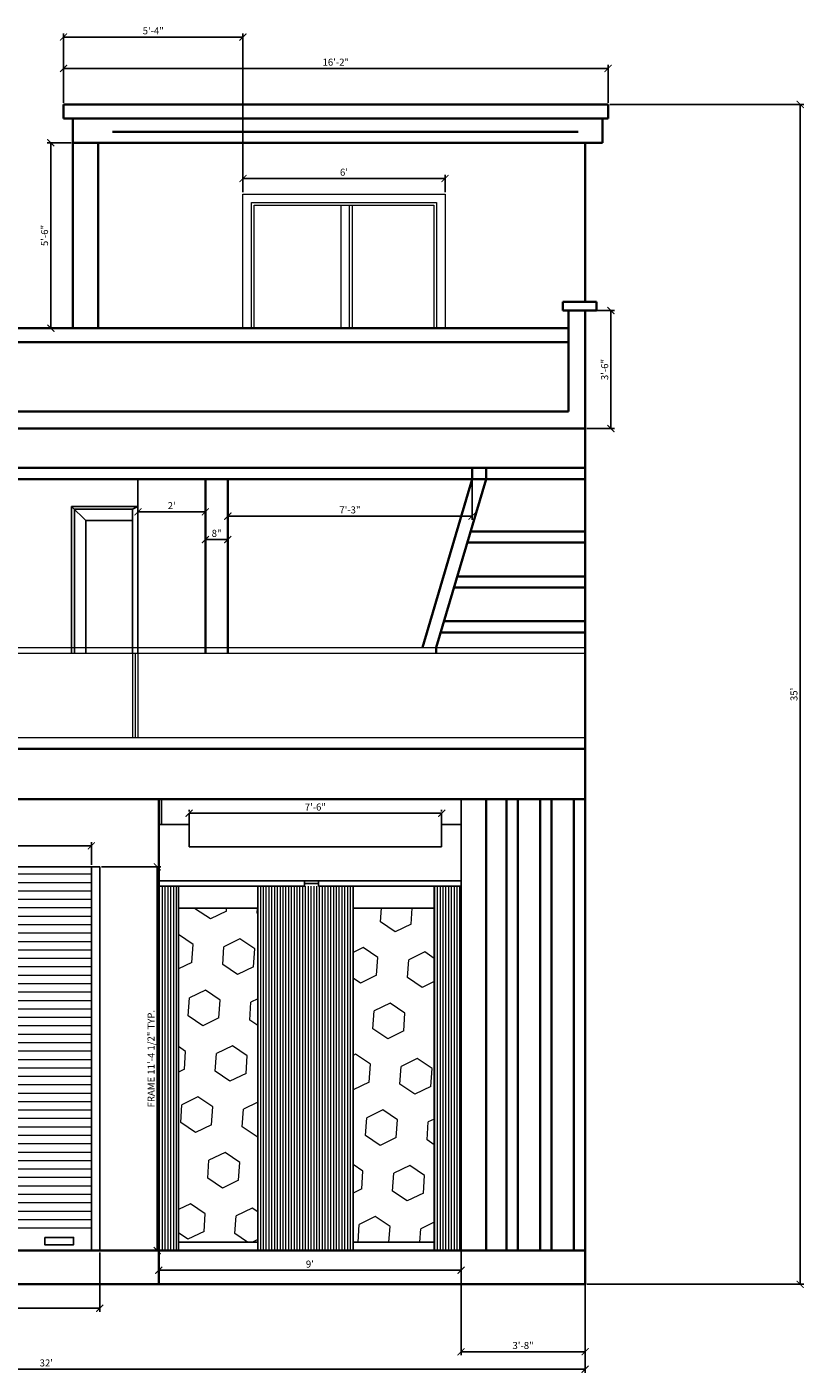
# Model space of a CAD drawing. Units: inches. Extents: x 3122 to 5933, y 1474 to 2995.
# Tile 2 of 12: x 3337 to 3614, y 1583 to 2063. Entities that reach past the tile are written whole.
import ezdxf

# ---------------------------------------------------------------- set-up
doc = ezdxf.new("R2010")
doc.units = ezdxf.units.IN
for name, color, linetype, lineweight in [('A-ANNO-DIMS', 2, 'Continuous', 18), ('A-ELEV', 7, 'Continuous', 35), ('A-ELEV-DOOR', 4, 'Continuous', 25), ('A-ELEV-GLAZ', 4, 'Continuous', 18), ('A-ELEV-PATT', 8, 'Continuous', 13), ('A-ELEV-RAIL', 7, 'Continuous', 18)]:
    doc.layers.add(name, color=color, linetype=linetype, lineweight=lineweight)
doc.styles.get("Standard").update_dxf_attribs({"font": 'arial.ttf'})
doc.dimstyles.new('ISO-25', dxfattribs={"dimtxt": 2.5, "dimasz": 2.5, "dimexe": 1.25, "dimexo": 0.625, "dimtad": 1, "dimdec": 0, "dimlunit": 3, "dimtxsty": 'Standard', "dimblk": 'ARCHTICK', "dimcen": 2.5, "dimadec": 0, "dimazin": 0, "dimtfac": 1, "dimtdec": 0, "dimtmove": 0, "dimatfit": 3, "dimfxl": 1, "dimarcsym": 0})

# ---------------------------------------------------------------- blocks, each defined once
blk = doc.blocks.new('_ArchTick')
at = {"color": 0, "linetype": 'ByBlock', "const_width": 0.15}
blk.add_lwpolyline([(-0.5, -0.5), (0.5, 0.5)], dxfattribs=at)
blk = doc.blocks.new('*D3')
at = {"layer": 'A-ANNO-DIMS', "color": 0, "lineweight": -2, "transparency": 16777216}
for p, q in [((3408.29, 1900.94), (3408.29, 1887.11)), ((3495.29, 1900.94), (3495.29, 1887.11)), ((3408.29, 1888.36), (3495.29, 1888.36))]:
    blk.add_line(p, q, dxfattribs=at)
at = {"layer": 'Defpoints', "color": 0, "transparency": 16777216}
for p in [(3408.29, 1901.56), (3495.29, 1901.56), (3495.29, 1888.36)]:
    blk.add_point(p, dxfattribs=at)
at = {"layer": 'A-ANNO-DIMS', "color": 0, "lineweight": -2, "transparency": 16777216, "xscale": 2.5, "yscale": 2.5, "zscale": 2.5, "rotation": 180}
blk.add_blockref('_ArchTick', (3408.29, 1888.36), dxfattribs=at)
at = {"layer": 'A-ANNO-DIMS', "color": 0, "lineweight": -2, "transparency": 16777216, "xscale": 2.5, "yscale": 2.5, "zscale": 2.5}
blk.add_blockref('_ArchTick', (3495.29, 1888.36), dxfattribs=at)
at = {"layer": 'A-ANNO-DIMS', "color": 0, "transparency": 16777216, "insert": (3451.79, 1890.26), "char_height": 2.5, "attachment_point": 5}
blk.add_mtext('7\'-3"', dxfattribs=at)
blk = doc.blocks.new('*D4')
at = {"layer": 'A-ANNO-DIMS', "color": 0, "lineweight": -2, "transparency": 16777216}
for p, q in [((3400.29, 1900.94), (3400.29, 1878.77)), ((3408.29, 1900.94), (3408.29, 1878.77)), ((3400.29, 1880.02), (3408.29, 1880.02))]:
    blk.add_line(p, q, dxfattribs=at)
at = {"layer": 'Defpoints', "color": 0, "transparency": 16777216}
for p in [(3400.29, 1901.56), (3408.29, 1901.56), (3408.29, 1880.02)]:
    blk.add_point(p, dxfattribs=at)
at = {"layer": 'A-ANNO-DIMS', "color": 0, "lineweight": -2, "transparency": 16777216, "xscale": 2.5, "yscale": 2.5, "zscale": 2.5, "rotation": 180}
blk.add_blockref('_ArchTick', (3400.29, 1880.02), dxfattribs=at)
at = {"layer": 'A-ANNO-DIMS', "color": 0, "lineweight": -2, "transparency": 16777216, "xscale": 2.5, "yscale": 2.5, "zscale": 2.5}
blk.add_blockref('_ArchTick', (3408.29, 1880.02), dxfattribs=at)
at = {"layer": 'A-ANNO-DIMS', "color": 0, "transparency": 16777216, "insert": (3404.29, 1881.92), "char_height": 2.5, "attachment_point": 5}
blk.add_mtext('8"', dxfattribs=at)
blk = doc.blocks.new('*D5')
at = {"layer": 'A-ANNO-DIMS', "color": 0, "lineweight": -2, "transparency": 16777216}
for p, q in [((3376.29, 1900.94), (3376.29, 1888.65)), ((3400.29, 1900.94), (3400.29, 1888.65)), ((3376.29, 1889.9), (3400.29, 1889.9))]:
    blk.add_line(p, q, dxfattribs=at)
at = {"layer": 'Defpoints', "color": 0, "transparency": 16777216}
for p in [(3376.29, 1901.56), (3400.29, 1901.56), (3400.29, 1889.9)]:
    blk.add_point(p, dxfattribs=at)
at = {"layer": 'A-ANNO-DIMS', "color": 0, "lineweight": -2, "transparency": 16777216, "xscale": 2.5, "yscale": 2.5, "zscale": 2.5, "rotation": 180}
blk.add_blockref('_ArchTick', (3376.29, 1889.9), dxfattribs=at)
at = {"layer": 'A-ANNO-DIMS', "color": 0, "lineweight": -2, "transparency": 16777216, "xscale": 2.5, "yscale": 2.5, "zscale": 2.5}
blk.add_blockref('_ArchTick', (3400.29, 1889.9), dxfattribs=at)
at = {"layer": 'A-ANNO-DIMS', "color": 0, "transparency": 16777216, "insert": (3388.29, 1891.78), "char_height": 2.5, "attachment_point": 5}
blk.add_mtext("2'", dxfattribs=at)
blk = doc.blocks.new('*D6')
at = {"layer": 'A-ANNO-DIMS', "color": 0, "lineweight": -2, "transparency": 16777216}
for p, q in [((3413.67, 2003.64), (3413.67, 2009.81)), ((3413.67, 2008.56), (3485.67, 2008.56)), ((3485.67, 2003.64), (3485.67, 2009.81))]:
    blk.add_line(p, q, dxfattribs=at)
at = {"layer": 'Defpoints', "color": 0, "transparency": 16777216}
for p in [(3485.67, 2008.56), (3413.67, 2003.02), (3485.67, 2003.02)]:
    blk.add_point(p, dxfattribs=at)
at = {"layer": 'A-ANNO-DIMS', "color": 0, "lineweight": -2, "transparency": 16777216, "xscale": 2.5, "yscale": 2.5, "zscale": 2.5, "rotation": 180}
blk.add_blockref('_ArchTick', (3413.67, 2008.56), dxfattribs=at)
at = {"layer": 'A-ANNO-DIMS', "color": 0, "lineweight": -2, "transparency": 16777216, "xscale": 2.5, "yscale": 2.5, "zscale": 2.5}
blk.add_blockref('_ArchTick', (3485.67, 2008.56), dxfattribs=at)
at = {"layer": 'A-ANNO-DIMS', "color": 0, "transparency": 16777216, "insert": (3449.67, 2010.46), "char_height": 2.5, "attachment_point": 5}
blk.add_mtext("6'", dxfattribs=at)
blk = doc.blocks.new('*D10')
at = {"layer": 'A-ANNO-DIMS', "color": 0, "lineweight": -2, "transparency": 16777216}
for p, q in [((3275.68, 1764.19), (3275.68, 1772.26)), ((3275.68, 1771.01), (3359.68, 1771.01)), ((3359.68, 1764.19), (3359.68, 1772.26))]:
    blk.add_line(p, q, dxfattribs=at)
at = {"layer": 'Defpoints', "color": 0, "transparency": 16777216}
for p in [(3359.68, 1771.01), (3275.68, 1763.56), (3359.68, 1763.56)]:
    blk.add_point(p, dxfattribs=at)
at = {"layer": 'A-ANNO-DIMS', "color": 0, "lineweight": -2, "transparency": 16777216, "xscale": 2.5, "yscale": 2.5, "zscale": 2.5, "rotation": 180}
blk.add_blockref('_ArchTick', (3275.68, 1771.01), dxfattribs=at)
at = {"layer": 'A-ANNO-DIMS', "color": 0, "lineweight": -2, "transparency": 16777216, "xscale": 2.5, "yscale": 2.5, "zscale": 2.5}
blk.add_blockref('_ArchTick', (3359.68, 1771.01), dxfattribs=at)
at = {"layer": 'A-ANNO-DIMS', "color": 0, "transparency": 16777216, "insert": (3317.68, 1772.89), "char_height": 2.5, "attachment_point": 5}
blk.add_mtext("7'", dxfattribs=at)
blk = doc.blocks.new('*D12')
at = {"layer": 'A-ANNO-DIMS', "color": 0, "lineweight": -2, "transparency": 16777216}
for p, q in [((3383.68, 1626.29), (3383.68, 1618.65)), ((3491.37, 1626.29), (3491.37, 1618.65)), ((3383.68, 1619.9), (3491.37, 1619.9))]:
    blk.add_line(p, q, dxfattribs=at)
at = {"layer": 'Defpoints', "color": 0, "transparency": 16777216}
for p in [(3383.68, 1626.92), (3491.37, 1626.92), (3491.37, 1619.9)]:
    blk.add_point(p, dxfattribs=at)
at = {"layer": 'A-ANNO-DIMS', "color": 0, "lineweight": -2, "transparency": 16777216, "xscale": 2.5, "yscale": 2.5, "zscale": 2.5, "rotation": 180}
blk.add_blockref('_ArchTick', (3383.68, 1619.9), dxfattribs=at)
at = {"layer": 'A-ANNO-DIMS', "color": 0, "lineweight": -2, "transparency": 16777216, "xscale": 2.5, "yscale": 2.5, "zscale": 2.5}
blk.add_blockref('_ArchTick', (3491.37, 1619.9), dxfattribs=at)
at = {"layer": 'A-ANNO-DIMS', "color": 0, "transparency": 16777216, "insert": (3437.52, 1621.8), "char_height": 2.5, "attachment_point": 5}
blk.add_mtext("9'", dxfattribs=at)
blk = doc.blocks.new('*D13')
at = {"layer": 'A-ANNO-DIMS', "color": 0, "lineweight": -2, "transparency": 16777216}
for p, q in [((3151.68, 1614.29), (3151.68, 1583.45)), ((3535.57, 1614.29), (3535.57, 1583.45)), ((3535.57, 1584.7), (3151.68, 1584.7))]:
    blk.add_line(p, q, dxfattribs=at)
at = {"layer": 'Defpoints', "color": 0, "transparency": 16777216}
for p in [(3151.68, 1614.92), (3535.57, 1614.92), (3151.68, 1584.7)]:
    blk.add_point(p, dxfattribs=at)
at = {"layer": 'A-ANNO-DIMS', "color": 0, "lineweight": -2, "transparency": 16777216, "xscale": 2.5, "yscale": 2.5, "zscale": 2.5, "rotation": 180}
blk.add_blockref('_ArchTick', (3151.68, 1584.7), dxfattribs=at)
at = {"layer": 'A-ANNO-DIMS', "color": 0, "lineweight": -2, "transparency": 16777216, "xscale": 2.5, "yscale": 2.5, "zscale": 2.5}
blk.add_blockref('_ArchTick', (3535.57, 1584.7), dxfattribs=at)
at = {"layer": 'A-ANNO-DIMS', "color": 0, "transparency": 16777216, "insert": (3343.62, 1586.6), "char_height": 2.5, "attachment_point": 5}
blk.add_mtext("32'", dxfattribs=at)
blk = doc.blocks.new('*D14')
at = {"layer": 'A-ANNO-DIMS', "color": 0, "lineweight": -2, "transparency": 16777216}
for p, q in [((3544.39, 2034.92), (3613.45, 2034.92)), ((3612.2, 1614.92), (3612.2, 2034.92)), ((3536.2, 1614.92), (3613.45, 1614.92))]:
    blk.add_line(p, q, dxfattribs=at)
at = {"layer": 'Defpoints', "color": 0, "transparency": 16777216}
for p in [(3543.76, 2034.92), (3612.2, 2034.92), (3535.57, 1614.92)]:
    blk.add_point(p, dxfattribs=at)
at = {"layer": 'A-ANNO-DIMS', "color": 0, "lineweight": -2, "transparency": 16777216, "xscale": 2.5, "yscale": 2.5, "zscale": 2.5}
for p, rotation in [((3612.2, 2034.92), 90), ((3612.2, 1614.92), 270)]:
    blk.add_blockref('_ArchTick', p, dxfattribs=dict(at, rotation=rotation))
at = {"layer": 'A-ANNO-DIMS', "color": 0, "transparency": 16777216, "insert": (3610.3, 1824.92), "char_height": 2.5, "attachment_point": 5, "rotation": 90}
blk.add_mtext("35'", dxfattribs=at)
blk = doc.blocks.new('*D16')
at = {"layer": 'A-ANNO-DIMS', "color": 0, "lineweight": -2, "transparency": 16777216}
for p, q in [((3349.76, 2035.54), (3349.76, 2049)), ((3349.76, 2047.75), (3543.76, 2047.75)), ((3543.76, 2035.54), (3543.76, 2049))]:
    blk.add_line(p, q, dxfattribs=at)
at = {"layer": 'Defpoints', "color": 0, "transparency": 16777216}
for p in [(3543.76, 2047.75), (3349.76, 2034.92), (3543.76, 2034.92)]:
    blk.add_point(p, dxfattribs=at)
at = {"layer": 'A-ANNO-DIMS', "color": 0, "lineweight": -2, "transparency": 16777216, "xscale": 2.5, "yscale": 2.5, "zscale": 2.5, "rotation": 180}
blk.add_blockref('_ArchTick', (3349.76, 2047.75), dxfattribs=at)
at = {"layer": 'A-ANNO-DIMS', "color": 0, "lineweight": -2, "transparency": 16777216, "xscale": 2.5, "yscale": 2.5, "zscale": 2.5}
blk.add_blockref('_ArchTick', (3543.76, 2047.75), dxfattribs=at)
at = {"layer": 'A-ANNO-DIMS', "color": 0, "transparency": 16777216, "insert": (3446.76, 2049.65), "char_height": 2.5, "attachment_point": 5}
blk.add_mtext('16\'-2"', dxfattribs=at)
blk = doc.blocks.new('*D17')
at = {"layer": 'A-ANNO-DIMS', "color": 0, "lineweight": -2, "transparency": 16777216}
for p, q in [((3352.48, 2021.27), (3343.99, 2021.27)), ((3345.24, 2021.27), (3345.24, 1955.27)), ((3352.48, 1955.27), (3343.99, 1955.27))]:
    blk.add_line(p, q, dxfattribs=at)
at = {"layer": 'Defpoints', "color": 0, "transparency": 16777216}
for p in [(3353.11, 2021.27), (3345.24, 1955.27), (3353.11, 1955.27)]:
    blk.add_point(p, dxfattribs=at)
at = {"layer": 'A-ANNO-DIMS', "color": 0, "lineweight": -2, "transparency": 16777216, "xscale": 2.5, "yscale": 2.5, "zscale": 2.5}
for p, rotation in [((3345.24, 2021.27), 90), ((3345.24, 1955.27), 270)]:
    blk.add_blockref('_ArchTick', p, dxfattribs=dict(at, rotation=rotation))
at = {"layer": 'A-ANNO-DIMS', "color": 0, "transparency": 16777216, "insert": (3343.33, 1988.27), "char_height": 2.5, "attachment_point": 5, "rotation": 90}
blk.add_mtext('5\'-6"', dxfattribs=at)
blk = doc.blocks.new('*D18')
at = {"layer": 'A-ANNO-DIMS', "color": 0, "lineweight": -2, "transparency": 16777216}
for p, q in [((3536.2, 1961.56), (3546.02, 1961.56)), ((3544.77, 1961.56), (3544.77, 1919.56)), ((3536.2, 1919.56), (3546.02, 1919.56))]:
    blk.add_line(p, q, dxfattribs=at)
at = {"layer": 'Defpoints', "color": 0, "transparency": 16777216}
for p in [(3535.57, 1961.56), (3535.57, 1919.56), (3544.77, 1919.56)]:
    blk.add_point(p, dxfattribs=at)
at = {"layer": 'A-ANNO-DIMS', "color": 0, "lineweight": -2, "transparency": 16777216, "xscale": 2.5, "yscale": 2.5, "zscale": 2.5}
for p, rotation in [((3544.77, 1961.56), 90), ((3544.77, 1919.56), 270)]:
    blk.add_blockref('_ArchTick', p, dxfattribs=dict(at, rotation=rotation))
at = {"layer": 'A-ANNO-DIMS', "color": 0, "transparency": 16777216, "insert": (3542.87, 1940.56), "char_height": 2.5, "attachment_point": 5, "rotation": 90}
blk.add_mtext('3\'-6"', dxfattribs=at)
blk = doc.blocks.new('*D21')
at = {"layer": 'A-ANNO-DIMS', "color": 0, "lineweight": -2, "transparency": 16777216}
for p, q in [((3394.47, 1783.22), (3394.47, 1783.84)), ((3484.47, 1783.22), (3484.47, 1783.84)), ((3394.47, 1782.59), (3484.47, 1782.59))]:
    blk.add_line(p, q, dxfattribs=at)
at = {"layer": 'Defpoints', "color": 0, "transparency": 16777216}
for p in [(3394.47, 1782.59), (3484.47, 1782.59), (3484.47, 1782.59)]:
    blk.add_point(p, dxfattribs=at)
at = {"layer": 'A-ANNO-DIMS', "color": 0, "lineweight": -2, "transparency": 16777216, "xscale": 2.5, "yscale": 2.5, "zscale": 2.5, "rotation": 180}
blk.add_blockref('_ArchTick', (3394.47, 1782.59), dxfattribs=at)
at = {"layer": 'A-ANNO-DIMS', "color": 0, "lineweight": -2, "transparency": 16777216, "xscale": 2.5, "yscale": 2.5, "zscale": 2.5}
blk.add_blockref('_ArchTick', (3484.47, 1782.59), dxfattribs=at)
at = {"layer": 'A-ANNO-DIMS', "color": 0, "transparency": 16777216, "insert": (3439.47, 1784.5), "char_height": 2.5, "attachment_point": 5}
blk.add_mtext('7\'-6"', dxfattribs=at)
blk = doc.blocks.new('SHUTTER-FRAME-84-ELEV')
for p, q in [((0, 136.64), (0, 0)), ((0, 136.64), (90, 136.64)), ((3, 136.64), (3, 0)), ((87, 136.64), (87, 0)), ((90, 136.64), (90, 0))]:
    blk.add_line(p, q)
blk = doc.blocks.new('SHUTTER-LIFT-PULL')
blk.add_lwpolyline([(0, 2.63), (10.24, 2.63), (10.24, 0), (0, 0)], close=True)
blk = doc.blocks.new('*D90')
at = {"layer": 'A-ANNO-DIMS', "color": 0, "lineweight": -2, "transparency": 16777216}
for p, q in [((3363.3, 1763.56), (3384.43, 1763.56)), ((3383.18, 1626.92), (3383.18, 1763.56)), ((3363.3, 1626.92), (3384.43, 1626.92))]:
    blk.add_line(p, q, dxfattribs=at)
at = {"layer": 'Defpoints', "color": 0, "transparency": 16777216}
for p in [(3362.68, 1763.56), (3383.18, 1763.56), (3362.68, 1626.92)]:
    blk.add_point(p, dxfattribs=at)
at = {"layer": 'A-ANNO-DIMS', "color": 0, "lineweight": -2, "transparency": 16777216, "xscale": 2.5, "yscale": 2.5, "zscale": 2.5}
for p, rotation in [((3383.18, 1763.56), 90), ((3383.18, 1626.92), 270)]:
    blk.add_blockref('_ArchTick', p, dxfattribs=dict(at, rotation=rotation))
at = {"layer": 'A-ANNO-DIMS', "color": 0, "transparency": 16777216, "insert": (3381.26, 1695.24), "char_height": 2.5, "attachment_point": 5, "rotation": 90}
blk.add_mtext('FRAME 11\'-4 1/2" TYP.', dxfattribs=at)
blk = doc.blocks.new('*D91')
at = {"layer": 'A-ANNO-DIMS', "color": 0, "lineweight": -2, "transparency": 16777216}
for p, q in [((3272.68, 1626.29), (3272.68, 1605.17)), ((3362.68, 1626.29), (3362.68, 1605.17)), ((3272.68, 1606.42), (3362.68, 1606.42))]:
    blk.add_line(p, q, dxfattribs=at)
at = {"layer": 'Defpoints', "color": 0, "transparency": 16777216}
for p in [(3272.68, 1626.92), (3362.68, 1626.92), (3362.68, 1606.42)]:
    blk.add_point(p, dxfattribs=at)
at = {"layer": 'A-ANNO-DIMS', "color": 0, "lineweight": -2, "transparency": 16777216, "xscale": 2.5, "yscale": 2.5, "zscale": 2.5, "rotation": 180}
blk.add_blockref('_ArchTick', (3272.68, 1606.42), dxfattribs=at)
at = {"layer": 'A-ANNO-DIMS', "color": 0, "lineweight": -2, "transparency": 16777216, "xscale": 2.5, "yscale": 2.5, "zscale": 2.5}
blk.add_blockref('_ArchTick', (3362.68, 1606.42), dxfattribs=at)
at = {"layer": 'A-ANNO-DIMS', "color": 0, "transparency": 16777216, "insert": (3317.68, 1608.32), "char_height": 2.5, "attachment_point": 5}
blk.add_mtext('7\'-6" TYP.', dxfattribs=at)
blk = doc.blocks.new('*D125')
at = {"layer": 'A-ANNO-DIMS', "color": 0, "lineweight": -2, "transparency": 16777216}
for p, q in [((3349.76, 2035.54), (3349.76, 2060.17)), ((3349.76, 2058.92), (3413.67, 2058.92)), ((3413.67, 2003.64), (3413.67, 2060.17))]:
    blk.add_line(p, q, dxfattribs=at)
at = {"layer": 'Defpoints', "color": 0, "transparency": 16777216}
for p in [(3413.67, 2058.92), (3349.76, 2034.92), (3413.67, 2003.02)]:
    blk.add_point(p, dxfattribs=at)
at = {"layer": 'A-ANNO-DIMS', "color": 0, "lineweight": -2, "transparency": 16777216, "xscale": 2.5, "yscale": 2.5, "zscale": 2.5, "rotation": 180}
blk.add_blockref('_ArchTick', (3349.76, 2058.92), dxfattribs=at)
at = {"layer": 'A-ANNO-DIMS', "color": 0, "lineweight": -2, "transparency": 16777216, "xscale": 2.5, "yscale": 2.5, "zscale": 2.5}
blk.add_blockref('_ArchTick', (3413.67, 2058.92), dxfattribs=at)
at = {"layer": 'A-ANNO-DIMS', "color": 0, "transparency": 16777216, "insert": (3381.72, 2060.82), "char_height": 2.5, "attachment_point": 5}
blk.add_mtext('5\'-4"', dxfattribs=at)
blk = doc.blocks.new('*D126')
at = {"layer": 'A-ANNO-DIMS', "color": 0, "lineweight": -2, "transparency": 16777216}
for p, q in [((3491.37, 1786.94), (3491.37, 1589.67)), ((3535.57, 1786.94), (3535.57, 1589.67)), ((3491.37, 1590.92), (3535.57, 1590.92))]:
    blk.add_line(p, q, dxfattribs=at)
at = {"layer": 'Defpoints', "color": 0, "transparency": 16777216}
for p in [(3491.37, 1787.56), (3535.57, 1787.56), (3535.57, 1590.92)]:
    blk.add_point(p, dxfattribs=at)
at = {"layer": 'A-ANNO-DIMS', "color": 0, "lineweight": -2, "transparency": 16777216, "xscale": 2.5, "yscale": 2.5, "zscale": 2.5, "rotation": 180}
blk.add_blockref('_ArchTick', (3491.37, 1590.92), dxfattribs=at)
at = {"layer": 'A-ANNO-DIMS', "color": 0, "lineweight": -2, "transparency": 16777216, "xscale": 2.5, "yscale": 2.5, "zscale": 2.5}
blk.add_blockref('_ArchTick', (3535.57, 1590.92), dxfattribs=at)
at = {"layer": 'A-ANNO-DIMS', "color": 0, "transparency": 16777216, "insert": (3513.47, 1592.82), "char_height": 2.5, "attachment_point": 5}
blk.add_mtext('3\'-8"', dxfattribs=at)

msp = doc.modelspace()

# ---------------------------------------------------------------- hatches: boundary and pattern name
at = {"layer": 'A-ELEV-PATT'}
h = msp.add_hatch(dxfattribs=at)
h.set_pattern_fill('ANSI31', color=256, scale=0.944882, angle=-45, style=0)
h.paths.add_polyline_path([(3275.68, 1634.07), (3359.68, 1634.07), (3359.68, 1763.05), (3275.68, 1763.05)])
h = msp.add_hatch(dxfattribs=at)
h.set_pattern_fill('ANSI31', color=256, scale=0.3149606, angle=45, style=0)
h.paths.add_polyline_path([(3383.68, 1626.92), (3390.68, 1626.92), (3390.68, 1756.59), (3383.68, 1756.59)])
h = msp.add_hatch(dxfattribs=at)
h.set_pattern_fill('ANSI31', color=256, scale=0.3149606, angle=45, style=0)
h.paths.add_polyline_path([(3418.96, 1626.92), (3452.91, 1626.92), (3452.91, 1756.59), (3418.96, 1756.59)])
h = msp.add_hatch(dxfattribs=at)
h.set_pattern_fill('ANSI31', color=256, scale=0.3149606, angle=45, style=0)
h.paths.add_polyline_path([(3481.86, 1626.92), (3491.37, 1626.92), (3491.37, 1756.59), (3481.86, 1756.59)])
h = msp.add_hatch(dxfattribs=at)
h.set_pattern_fill('HEX', color=256, scale=2, angle=86)
h.paths.add_polyline_path([(3418.96, 1748.78), (3390.68, 1748.78), (3390.68, 1629.92), (3418.96, 1629.92)])
h.paths.add_polyline_path([(3481.86, 1748.78), (3452.91, 1748.78), (3452.91, 1629.92), (3481.86, 1629.92)])

# ---------------------------------------------------------------- linework, layer by layer
at = {"layer": 'A-ELEV'}
for p, q in [((3349.76, 2034.92), (3543.76, 2034.92)), ((3349.76, 2029.92), (3349.76, 2034.92)), ((3543.76, 2029.92), (3543.76, 2034.92)), ((3349.76, 2029.92), (3543.76, 2029.92)), ((3353.11, 2029.92), (3353.11, 2021.27)), ((3541.74, 2021.27), (3541.74, 2029.92)), ((3367.16, 2025.16), (3533.16, 2025.16)), ((3353.11, 2021.27), (3541.74, 2021.27)), ((3353.11, 2021.27), (3353.11, 1955.27)), ((3362.11, 2021.27), (3362.11, 1955.27)), ((3535.57, 2021.27), (3535.57, 1964.61)), ((3539.63, 1964.61), (3527.63, 1964.61)), ((3527.63, 1961.56), (3527.63, 1964.61)), ((3539.63, 1961.56), (3527.63, 1961.56)), ((3529.68, 1961.56), (3529.68, 1925.56)), ((3535.57, 1961.56), (3535.57, 1919.56)), ((3539.63, 1964.61), (3539.63, 1961.56)), ((3353.11, 1955.27), (3327.58, 1955.27)), ((3353.11, 1955.27), (3529.68, 1955.27)), ((3327.58, 1950.27), (3353.11, 1950.27)), ((3353.11, 1950.27), (3529.68, 1950.27)), ((3529.68, 1925.56), (3151.68, 1925.56)), ((3535.57, 1919.56), (3151.68, 1919.56)), ((3535.57, 1919.56), (3535.57, 1614.92)), ((3535.57, 1905.56), (3171.68, 1905.56)), ((3495.29, 1901.56), (3495.29, 1905.56)), ((3500.29, 1901.56), (3500.29, 1905.56)), ((3535.57, 1901.56), (3175.68, 1901.56)), ((3400.29, 1901.56), (3400.29, 1839.56)), ((3408.29, 1901.56), (3408.29, 1839.56)), ((3495.29, 1901.56), (3477.59, 1841.56)), ((3500.29, 1901.56), (3482.5, 1841.56)), ((3493.58, 1878.94), (3535.57, 1878.94)), ((3494.77, 1882.94), (3535.57, 1882.94)), ((3490.02, 1866.94), (3535.57, 1866.94)), ((3488.84, 1862.94), (3535.57, 1862.94)), ((3485.28, 1850.94), (3535.57, 1850.94)), ((3484.09, 1846.94), (3535.57, 1846.94)), ((3482.5, 1841.56), (3482.5, 1839.56)), ((3175.68, 1805.56), (3535.57, 1805.56)), ((3151.68, 1787.56), (3535.57, 1787.56)), ((3383.68, 1787.56), (3383.68, 1614.92)), ((3500.37, 1787.56), (3500.37, 1626.92)), ((3507.57, 1787.56), (3507.57, 1626.92)), ((3511.57, 1787.56), (3511.57, 1626.92)), ((3519.57, 1787.56), (3519.57, 1626.92)), ((3523.57, 1787.56), (3523.57, 1626.92)), ((3531.57, 1787.56), (3531.57, 1626.92)), ((3151.68, 1626.92), (3535.57, 1626.92)), ((3151.68, 1614.92), (3535.57, 1614.92))]:
    msp.add_line(p, q, dxfattribs=at)
at = {"layer": 'A-ELEV-DOOR'}
for p, q in [((3376.29, 1901.56), (3376.29, 1839.56)), ((3352.65, 1839.56), (3352.65, 1891.83)), ((3352.65, 1891.83), (3376.29, 1891.83)), ((3352.65, 1891.83), (3357.65, 1886.83)), ((3353.65, 1890.83), (3374.29, 1890.83)), ((3353.65, 1839.56), (3353.65, 1890.83)), ((3374.29, 1890.83), (3376.29, 1891.83)), ((3374.29, 1890.83), (3374.29, 1839.56)), ((3357.65, 1839.56), (3357.65, 1886.83)), ((3357.65, 1886.83), (3374.29, 1886.83)), ((3384.68, 1787.56), (3384.68, 1778.56)), ((3491.37, 1787.56), (3491.37, 1626.92)), ((3383.68, 1778.56), (3394.47, 1778.56)), ((3394.47, 1778.56), (3394.47, 1782.59)), ((3394.47, 1782.59), (3484.47, 1782.59)), ((3394.47, 1770.59), (3394.47, 1778.56)), ((3484.47, 1782.59), (3484.47, 1770.59)), ((3484.47, 1778.56), (3491.37, 1778.56)), ((3394.47, 1770.59), (3484.47, 1770.59)), ((3383.68, 1758.59), (3491.37, 1758.59)), ((3383.68, 1756.59), (3435.56, 1756.59)), ((3390.68, 1756.59), (3390.68, 1626.92)), ((3418.96, 1756.59), (3418.96, 1626.92)), ((3435.56, 1756.59), (3435.56, 1758.59)), ((3435.56, 1757.61), (3440.56, 1757.61)), ((3440.56, 1756.59), (3440.56, 1758.59)), ((3440.56, 1756.59), (3491.37, 1756.59)), ((3452.91, 1756.59), (3452.91, 1626.92)), ((3481.86, 1756.59), (3481.86, 1626.92)), ((3418.96, 1748.78), (3390.68, 1748.78)), ((3452.91, 1748.78), (3481.86, 1748.78)), ((3390.68, 1629.92), (3418.96, 1629.92)), ((3452.91, 1629.92), (3481.86, 1629.92))]:
    msp.add_line(p, q, dxfattribs=at)
at = {"layer": 'A-ELEV-GLAZ'}
for p, q in [((3413.67, 1955.27), (3413.67, 2003.02)), ((3413.67, 2003.02), (3485.67, 2003.02)), ((3416.67, 2000.02), (3482.67, 2000.02)), ((3416.67, 1955.27), (3416.67, 2000.02)), ((3417.67, 1955.27), (3417.67, 1999.02)), ((3417.67, 1999.02), (3481.67, 1999.02)), ((3448.54, 1999.02), (3448.54, 1955.27)), ((3451.54, 1999.02), (3451.54, 1955.27)), ((3452.54, 1999.02), (3452.54, 1955.27)), ((3481.67, 1999.02), (3481.67, 1955.27)), ((3482.67, 2000.02), (3482.67, 1955.27)), ((3485.67, 2003.02), (3485.67, 1955.27))]:
    msp.add_line(p, q, dxfattribs=at)
at = {"layer": 'A-ELEV-RAIL'}
for p, q in [((3175.68, 1841.56), (3535.57, 1841.56)), ((3235.68, 1839.56), (3535.57, 1839.56)), ((3374.29, 1839.56), (3374.29, 1809.56)), ((3375.29, 1839.56), (3375.29, 1809.56)), ((3376.29, 1839.56), (3376.29, 1809.56)), ((3240.68, 1809.56), (3535.57, 1809.56))]:
    msp.add_line(p, q, dxfattribs=at)

# ---------------------------------------------------------------- block references
at = {"layer": 'A-ELEV-DOOR'}
for name, p in [('SHUTTER-FRAME-84-ELEV', (3272.68, 1626.92)), ('SHUTTER-LIFT-PULL', (3343.09, 1628.97))]:
    msp.add_blockref(name, p, dxfattribs=at)

# ---------------------------------------------------------------- dimensions: what is measured, and where the dimension line sits
at = {"layer": 'A-ANNO-DIMS'}
for base, p1, p2, override, picture, middle in [((3413.67, 2058.92), (3349.76, 2034.92), (3413.67, 2003.02), {"dimdec": 1, "dimlfac": 1, "dimrnd": 0, "dimzin": 1, "dimdsep": 46, "dimlunit": 4, "dimfrac": 2}, '*D125', (3381.72, 2060.82)), ((3543.76, 2047.75), (3349.76, 2034.92), (3543.76, 2034.92), {"dimclrd": 0, "dimclre": 0, "dimclrt": 0}, '*D16', (3446.76, 2049.65)), ((3485.67, 2008.56), (3413.67, 2003.02), (3485.67, 2003.02), {"dimclrd": 0, "dimclre": 0, "dimclrt": 0}, '*D6', (3449.67, 2010.46)), ((3400.29, 1889.9), (3376.29, 1901.56), (3400.29, 1901.56), {"dimclrd": 0, "dimclre": 0, "dimclrt": 0}, '*D5', (3388.29, 1891.78)), ((3408.29, 1880.02), (3400.29, 1901.56), (3408.29, 1901.56), {"dimclrd": 0, "dimclre": 0, "dimclrt": 0}, '*D4', (3404.29, 1881.92)), ((3495.29, 1888.36), (3408.29, 1901.56), (3495.29, 1901.56), {"dimclrd": 0, "dimclre": 0, "dimclrt": 0}, '*D3', (3451.79, 1890.26)), ((3535.57, 1590.92), (3491.37, 1787.56), (3535.57, 1787.56), {"dimdec": 1, "dimlfac": 1, "dimrnd": 0, "dimzin": 1, "dimdsep": 46, "dimlunit": 4, "dimfrac": 2}, '*D126', (3513.47, 1592.82)), ((3484.47, 1782.59), (3394.47, 1782.59), (3484.47, 1782.59), {"dimclrd": 0, "dimclre": 0, "dimclrt": 0}, '*D21', (3439.47, 1784.5)), ((3359.68, 1771.01), (3275.68, 1763.56), (3359.68, 1763.56), {"dimclrd": 0, "dimclre": 0, "dimclrt": 0}, '*D10', (3317.68, 1772.89)), ((3491.37, 1619.9), (3383.68, 1626.92), (3491.37, 1626.92), {"dimclrd": 0, "dimclre": 0, "dimclrt": 0}, '*D12', (3437.52, 1621.8)), ((3151.68, 1584.7), (3535.57, 1614.92), (3151.68, 1614.92), {"dimclrd": 0, "dimclre": 0, "dimclrt": 0}, '*D13', (3343.62, 1586.6))]:
    dim = msp.add_linear_dim(base=base, p1=p1, p2=p2, dimstyle='ISO-25', override=override, dxfattribs=at)
    dim.commit()
    dim.dimension.update_dxf_attribs({"geometry": picture, "text_midpoint": middle})
for base, p1, p2, picture, middle in [((3612.2, 2034.92), (3535.57, 1614.92), (3543.76, 2034.92), '*D14', (3610.3, 1824.92)), ((3345.24, 1955.27), (3353.11, 2021.27), (3353.11, 1955.27), '*D17', (3343.33, 1988.27)), ((3544.77, 1919.56), (3535.57, 1961.56), (3535.57, 1919.56), '*D18', (3542.87, 1940.56))]:
    dim = msp.add_linear_dim(base=base, p1=p1, p2=p2, angle=90, dimstyle='ISO-25', override={"dimclrd": 0, "dimclre": 0, "dimclrt": 0}, dxfattribs=at)
    dim.commit()
    dim.dimension.update_dxf_attribs({"geometry": picture, "text_midpoint": middle})
dim = msp.add_linear_dim(base=(3383.18, 1763.56), p1=(3362.68, 1626.92), p2=(3362.68, 1763.56), angle=90, text='FRAME <> TYP.', dimstyle='ISO-25', override={"dimdec": 1, "dimlfac": 1, "dimrnd": 0, "dimzin": 1, "dimdsep": 46, "dimlunit": 4, "dimfrac": 2}, dxfattribs=at)
dim.commit()
dim.dimension.update_dxf_attribs({"geometry": '*D90', "text_midpoint": (3381.26, 1695.24)})
dim = msp.add_linear_dim(base=(3362.68, 1606.42), p1=(3272.68, 1626.92), p2=(3362.68, 1626.92), text='<> TYP.', dimstyle='ISO-25', override={"dimdec": 1, "dimlfac": 1, "dimrnd": 0, "dimzin": 1, "dimdsep": 46, "dimlunit": 4, "dimfrac": 2}, dxfattribs=at)
dim.commit()
dim.dimension.update_dxf_attribs({"geometry": '*D91', "text_midpoint": (3317.68, 1608.32)})

doc.saveas('drawing.dxf')
